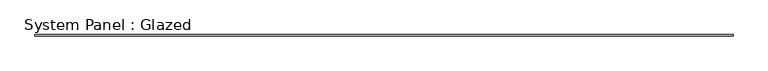
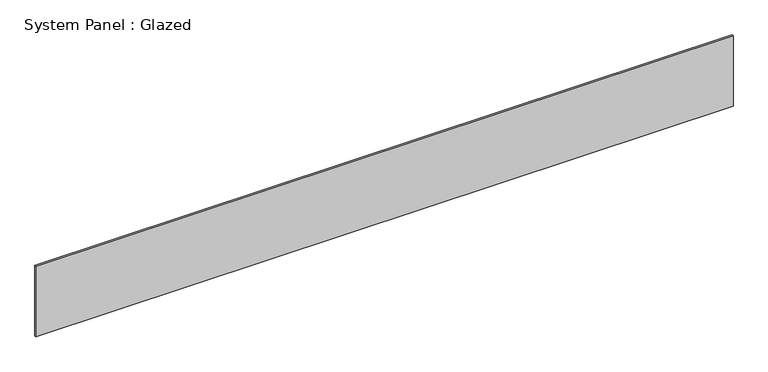
"""IFC4 building model written with IfcOpenShell, lengths in millimetres: plate geometry, System Panel : Glazed."""

from ifc_helpers import new_model, si_unit, origin, origin_with_axes, place, context, project, spatial, polyline, outline, extrude, source, transform, mapped, element, save


def system_panel_glazed_f332d308(model_context):
    return source(origin(), model_context, "Body", "SweptSolid", [
        extrude(outline(polyline([(6825.385375, 19.05), (-6825.385375, 19.05), (-6825.385375, 44.45), (6825.385375, 44.45), (6825.385375, 19.05)])), origin_with_axes(), (0.0, 0.0, 1.0), 1460.5),
    ])


if __name__ == "__main__":
    model = new_model("IFC4")
    model_context = context("Model", 3, world=origin())
    ifc_project = project(units=[si_unit("LENGTHUNIT", "METRE", prefix="MILLI")], contexts=[model_context])
    site = spatial("IfcSite", under=ifc_project)
    building = spatial("IfcBuilding", under=site)
    placement = place(None, origin())
    system_panel_glazed_shape = system_panel_glazed_f332d308(model_context)
    element("IfcPlate", 1, ObjectType="System Panel : Glazed", at=placement, inside=building, context=model_context, shape_type="MappedRepresentation", body=[
        mapped(system_panel_glazed_shape, transform((0.0, 0.0, 0.0), x_axis=(1.0, 0.0, 0.0), y_axis=(0.0, 1.0, 0.0), z_axis=(0.0, 0.0, 1.0))),
    ])
    save(model, "model.ifc")

# Revit data of these elements
# Type "System Panel : Glazed"
#   Construction Type Id = "GSP4R"
#   Analytic Construction = "1/8 in Pilkington single glazing"
#   Visual Light Transmittance = 0.9
#   Solar Heat Gain Coefficient = 0.86
#   Heat Transfer Coefficient (U) = 1.18115 BTU/(h·ft²·°F)
# Element 1 (IfcPlate, "System Panel : Glazed")
#   Materials on its faces: "Glass"
# Materials
#   "Glass": class "Glass", colour RGB 0 128 192, transparency 0.75, Description = "Soda Lime Glass", Cost = 0
